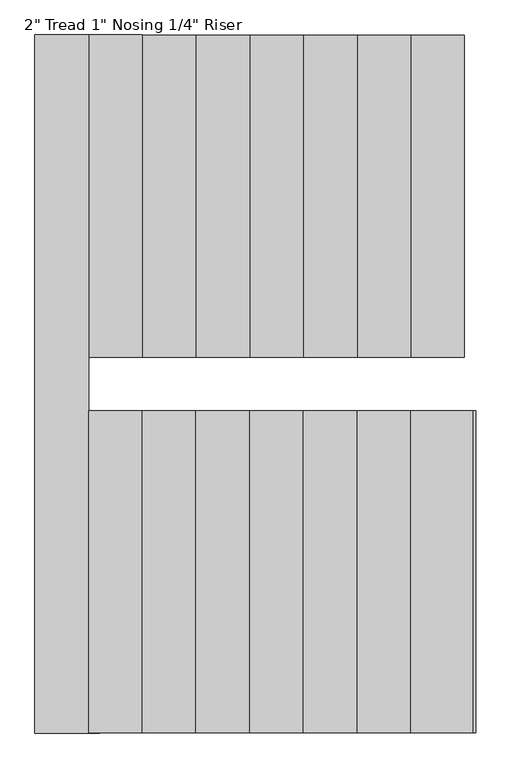
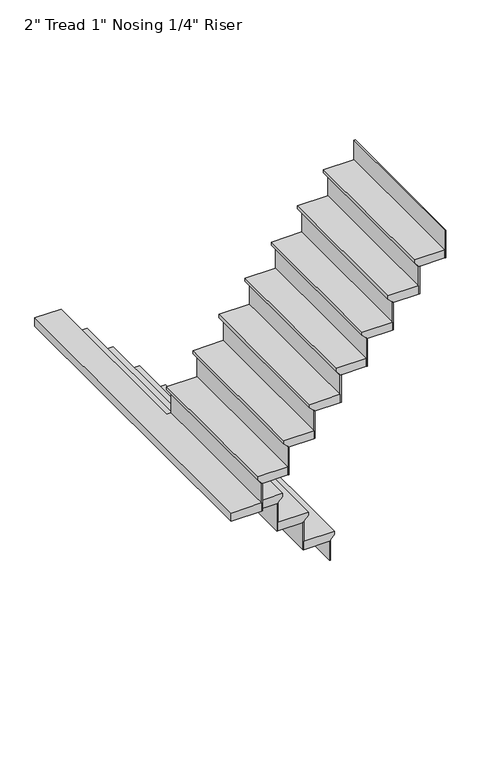
"""IFC4 building model written with IfcOpenShell, lengths in millimetres: stair flight geometry."""

from ifc_helpers import new_model, si_unit, origin, place, context, project, spatial, faceted_brep, source, transform, mapped, element, save


def stair_flight_9f5b5764(model_context):
    return source(origin(), model_context, "Body", "Brep", [
        faceted_brep([(3632.2, 10909.3, 9294.2833333), (3632.2, 10909.3, 9313.3333333), (3632.2, 9994.9, 9313.3333333), (3632.2, 9994.9, 9294.2833333), (3606.8, 10909.3, 9268.8833333), (3606.8, 9994.9, 9268.8833333), (3454.4, 10909.3, 9313.3333333), (3454.4, 9994.9, 9313.3333333), (3606.8, 9994.9, 9262.5333333), (3454.4, 9994.9, 9262.5333333), (3454.4, 10909.3, 9262.5333333), (3606.8, 10909.3, 9262.5333333)], [[[0, 1, 2, 3]], [[4, 0, 3, 5]], [[2, 1, 6, 7]], [[8, 9, 10, 11]], [[2, 7, 9, 8, 5, 3]], [[8, 11, 4, 5]], [[6, 1, 0, 4, 11, 10]], [[7, 6, 10, 9]]]),
        faceted_brep([(3606.8, 10909.3, 9262.5333333), (3606.8, 10909.3, 9144.0), (3600.45, 10909.3, 9144.0), (3600.45, 10909.3, 9262.5333333), (3606.8, 9994.9, 9262.5333333), (3600.45, 9994.9, 9262.5333333), (3600.45, 9994.9, 9144.0), (3606.8, 9994.9, 9144.0)], [[[0, 1, 2, 3]], [[4, 5, 6, 7]], [[1, 0, 4, 7]], [[2, 1, 7, 6]], [[3, 2, 6, 5]], [[0, 3, 5, 4]]]),
        faceted_brep([(3454.4, 10909.3, 9431.8666667), (3454.4, 10909.3, 9262.5333333), (3448.05, 10909.3, 9262.5333333), (3448.05, 10909.3, 9431.8666667), (3454.4, 9994.9, 9431.8666667), (3448.05, 9994.9, 9431.8666667), (3448.05, 9994.9, 9262.5333333), (3454.4, 9994.9, 9262.5333333)], [[[0, 1, 2, 3]], [[4, 5, 6, 7]], [[1, 0, 4, 7]], [[2, 1, 7, 6]], [[3, 2, 6, 5]], [[0, 3, 5, 4]]]),
        faceted_brep([(3479.8, 9994.9, 9482.6666667), (3479.8, 10909.3, 9482.6666667), (3302.0, 10909.3, 9482.6666667), (3302.0, 9994.9, 9482.6666667), (3454.4, 9994.9, 9431.8666667), (3302.0, 9994.9, 9431.8666667), (3302.0, 10909.3, 9431.8666667), (3454.4, 10909.3, 9431.8666667), (3454.4, 9994.9, 9438.2166667), (3479.8, 9994.9, 9463.6166667), (3454.4, 10909.3, 9438.2166667), (3479.8, 10909.3, 9463.6166667)], [[[0, 1, 2, 3]], [[4, 5, 6, 7]], [[0, 3, 5, 4, 8, 9]], [[4, 7, 10, 8]], [[2, 1, 11, 10, 7, 6]], [[3, 2, 6, 5]], [[11, 1, 0, 9]], [[10, 11, 9, 8]]]),
        faceted_brep([(3302.0, 10909.3, 9601.2), (3302.0, 10909.3, 9431.8666667), (3295.65, 10909.3, 9431.8666667), (3295.65, 10909.3, 9601.2), (3302.0, 9994.9, 9601.2), (3295.65, 9994.9, 9601.2), (3295.65, 9994.9, 9431.8666667), (3302.0, 9994.9, 9431.8666667)], [[[0, 1, 2, 3]], [[4, 5, 6, 7]], [[1, 0, 4, 7]], [[2, 1, 7, 6]], [[3, 2, 6, 5]], [[0, 3, 5, 4]]]),
        faceted_brep([(3327.4, 9994.9, 9652.0), (3327.4, 10909.3, 9652.0), (3149.6, 10909.3, 9652.0), (3149.6, 9994.9, 9652.0), (3302.0, 9994.9, 9601.2), (3149.6, 9994.9, 9601.2), (3149.6, 10909.3, 9601.2), (3302.0, 10909.3, 9601.2), (3302.0, 9994.9, 9607.55), (3327.4, 9994.9, 9632.95), (3302.0, 10909.3, 9607.55), (3327.4, 10909.3, 9632.95)], [[[0, 1, 2, 3]], [[4, 5, 6, 7]], [[0, 3, 5, 4, 8, 9]], [[4, 7, 10, 8]], [[2, 1, 11, 10, 7, 6]], [[3, 2, 6, 5]], [[11, 1, 0, 9]], [[10, 11, 9, 8]]]),
        faceted_brep([(3149.6, 10909.3, 9770.5333333), (3149.6, 10909.3, 9601.2), (3143.25, 10909.3, 9601.2), (3143.25, 10909.3, 9770.5333333), (3149.6, 9994.9, 9770.5333333), (3143.25, 9994.9, 9770.5333333), (3143.25, 9994.9, 9601.2), (3149.6, 9994.9, 9601.2)], [[[0, 1, 2, 3]], [[4, 5, 6, 7]], [[1, 0, 4, 7]], [[2, 1, 7, 6]], [[3, 2, 6, 5]], [[0, 3, 5, 4]]]),
        faceted_brep([(3175.0, 9994.9, 9821.3333333), (3175.0, 10909.3, 9821.3333333), (2997.2, 10909.3, 9821.3333333), (2997.2, 9994.9, 9821.3333333), (3149.6, 9994.9, 9770.5333333), (2997.2, 9994.9, 9770.5333333), (2997.2, 10909.3, 9770.5333333), (3149.6, 10909.3, 9770.5333333), (3149.6, 9994.9, 9776.8833333), (3175.0, 9994.9, 9802.2833333), (3149.6, 10909.3, 9776.8833333), (3175.0, 10909.3, 9802.2833333)], [[[0, 1, 2, 3]], [[4, 5, 6, 7]], [[0, 3, 5, 4, 8, 9]], [[4, 7, 10, 8]], [[2, 1, 11, 10, 7, 6]], [[3, 2, 6, 5]], [[11, 1, 0, 9]], [[10, 11, 9, 8]]]),
        faceted_brep([(2997.2, 10909.3, 9939.8666667), (2997.2, 10909.3, 9770.5333333), (2990.85, 10909.3, 9770.5333333), (2990.85, 10909.3, 9939.8666667), (2997.2, 9994.9, 9939.8666667), (2990.85, 9994.9, 9939.8666667), (2990.85, 9994.9, 9770.5333333), (2997.2, 9994.9, 9770.5333333)], [[[0, 1, 2, 3]], [[4, 5, 6, 7]], [[1, 0, 4, 7]], [[2, 1, 7, 6]], [[3, 2, 6, 5]], [[0, 3, 5, 4]]]),
        faceted_brep([(3022.6, 9994.9, 9990.6666667), (3022.6, 10909.3, 9990.6666667), (2844.8, 10909.3, 9990.6666667), (2844.8, 9994.9, 9990.6666667), (2997.2, 9994.9, 9939.8666667), (2844.8, 9994.9, 9939.8666667), (2844.8, 10909.3, 9939.8666667), (2997.2, 10909.3, 9939.8666667), (2997.2, 9994.9, 9946.2166667), (3022.6, 9994.9, 9971.6166667), (2997.2, 10909.3, 9946.2166667), (3022.6, 10909.3, 9971.6166667)], [[[0, 1, 2, 3]], [[4, 5, 6, 7]], [[0, 3, 5, 4, 8, 9]], [[4, 7, 10, 8]], [[2, 1, 11, 10, 7, 6]], [[3, 2, 6, 5]], [[11, 1, 0, 9]], [[10, 11, 9, 8]]]),
        faceted_brep([(2844.8, 10909.3, 10109.2), (2844.8, 10909.3, 9939.8666667), (2838.45, 10909.3, 9939.8666667), (2838.45, 10909.3, 10109.2), (2844.8, 9994.9, 10109.2), (2838.45, 9994.9, 10109.2), (2838.45, 9994.9, 9939.8666667), (2844.8, 9994.9, 9939.8666667)], [[[0, 1, 2, 3]], [[4, 5, 6, 7]], [[1, 0, 4, 7]], [[2, 1, 7, 6]], [[3, 2, 6, 5]], [[0, 3, 5, 4]]]),
        faceted_brep([(2870.2, 9994.9, 10160.0), (2870.2, 10909.3, 10160.0), (2692.4, 10909.3, 10160.0), (2692.4, 9994.9, 10160.0), (2844.8, 9994.9, 10109.2), (2692.4, 9994.9, 10109.2), (2692.4, 10909.3, 10109.2), (2844.8, 10909.3, 10109.2), (2844.8, 9994.9, 10115.55), (2870.2, 9994.9, 10140.95), (2844.8, 10909.3, 10115.55), (2870.2, 10909.3, 10140.95)], [[[0, 1, 2, 3]], [[4, 5, 6, 7]], [[0, 3, 5, 4, 8, 9]], [[4, 7, 10, 8]], [[2, 1, 11, 10, 7, 6]], [[3, 2, 6, 5]], [[11, 1, 0, 9]], [[10, 11, 9, 8]]]),
        faceted_brep([(2692.4, 10909.3, 10278.5333333), (2692.4, 10909.3, 10109.2), (2686.05, 10909.3, 10109.2), (2686.05, 10909.3, 10278.5333333), (2692.4, 9994.9, 10278.5333333), (2686.05, 9994.9, 10278.5333333), (2686.05, 9994.9, 10109.2), (2692.4, 9994.9, 10109.2)], [[[0, 1, 2, 3]], [[4, 5, 6, 7]], [[1, 0, 4, 7]], [[2, 1, 7, 6]], [[3, 2, 6, 5]], [[0, 3, 5, 4]]]),
        faceted_brep([(2717.8, 9994.9, 10329.3333333), (2717.8, 10909.3, 10329.3333333), (2540.0, 10909.3, 10329.3333333), (2540.0, 9994.9, 10329.3333333), (2692.4, 9994.9, 10278.5333333), (2540.0, 9994.9, 10278.5333333), (2540.0, 10909.3, 10278.5333333), (2692.4, 10909.3, 10278.5333333), (2692.4, 9994.9, 10284.8833333), (2717.8, 9994.9, 10310.2833333), (2692.4, 10909.3, 10284.8833333), (2717.8, 10909.3, 10310.2833333)], [[[0, 1, 2, 3]], [[4, 5, 6, 7]], [[0, 3, 5, 4, 8, 9]], [[4, 7, 10, 8]], [[2, 1, 11, 10, 7, 6]], [[3, 2, 6, 5]], [[11, 1, 0, 9]], [[10, 11, 9, 8]]]),
        faceted_brep([(2540.0, 10909.3, 10447.8666667), (2540.0, 10909.3, 10278.5333333), (2533.65, 10909.3, 10278.5333333), (2533.65, 10909.3, 10447.8666667), (2540.0, 9994.9, 10447.8666667), (2533.65, 9994.9, 10447.8666667), (2533.65, 9994.9, 10278.5333333), (2540.0, 9994.9, 10278.5333333)], [[[0, 1, 2, 3]], [[4, 5, 6, 7]], [[1, 0, 4, 7]], [[2, 1, 7, 6]], [[3, 2, 6, 5]], [[0, 3, 5, 4]]]),
        faceted_brep([(2590.8, 9842.5, 10498.6666667), (2565.4, 9842.5, 10498.6666667), (2565.4, 10909.3, 10498.6666667), (2413.0, 10909.3, 10498.6666667), (2413.0, 8928.1, 10498.6666667), (2590.8, 8928.1, 10498.6666667), (2565.4, 9842.5, 10447.8666667), (2590.8, 9842.5, 10447.8666667), (2590.8, 8928.1, 10447.8666667), (2413.0, 8928.1, 10447.8666667), (2413.0, 10909.3, 10447.8666667), (2540.0, 10909.3, 10447.8666667), (2540.0, 9994.9, 10447.8666667), (2565.4, 9994.9, 10447.8666667), (2565.4, 9994.9, 10479.6166667), (2565.4, 10909.3, 10479.6166667), (2540.0, 9994.9, 10454.2166667), (2540.0, 10909.3, 10454.2166667)], [[[0, 1, 2, 3, 4, 5]], [[6, 7, 8, 9, 10, 11, 12, 13]], [[1, 0, 7, 6]], [[2, 1, 6, 13, 14, 15]], [[13, 12, 16, 14]], [[12, 11, 17, 16]], [[3, 2, 15, 17, 11, 10]], [[4, 3, 10, 9]], [[5, 4, 9, 8]], [[0, 5, 8, 7]], [[17, 15, 14, 16]]]),
        faceted_brep([(2590.8, 8928.1, 10617.2), (2590.8, 8928.1, 10447.8666667), (2597.15, 8928.1, 10447.8666667), (2597.15, 8928.1, 10617.2), (2590.8, 9842.5, 10617.2), (2597.15, 9842.5, 10617.2), (2597.15, 9842.5, 10447.8666667), (2590.8, 9842.5, 10447.8666667)], [[[0, 1, 2, 3]], [[4, 5, 6, 7]], [[1, 0, 4, 7]], [[2, 1, 7, 6]], [[3, 2, 6, 5]], [[0, 3, 5, 4]]]),
        faceted_brep([(2565.4, 9842.5, 10668.0), (2565.4, 8928.1, 10668.0), (2743.2, 8928.1, 10668.0), (2743.2, 9842.5, 10668.0), (2590.8, 9842.5, 10617.2), (2743.2, 9842.5, 10617.2), (2743.2, 8928.1, 10617.2), (2590.8, 8928.1, 10617.2), (2590.8, 9842.5, 10623.55), (2565.4, 9842.5, 10648.95), (2590.8, 8928.1, 10623.55), (2565.4, 8928.1, 10648.95)], [[[0, 1, 2, 3]], [[4, 5, 6, 7]], [[0, 3, 5, 4, 8, 9]], [[4, 7, 10, 8]], [[2, 1, 11, 10, 7, 6]], [[3, 2, 6, 5]], [[11, 1, 0, 9]], [[10, 11, 9, 8]]]),
        faceted_brep([(2743.2, 8928.1, 10786.5333333), (2743.2, 8928.1, 10617.2), (2749.55, 8928.1, 10617.2), (2749.55, 8928.1, 10786.5333333), (2743.2, 9842.5, 10786.5333333), (2749.55, 9842.5, 10786.5333333), (2749.55, 9842.5, 10617.2), (2743.2, 9842.5, 10617.2)], [[[0, 1, 2, 3]], [[4, 5, 6, 7]], [[1, 0, 4, 7]], [[2, 1, 7, 6]], [[3, 2, 6, 5]], [[0, 3, 5, 4]]]),
        faceted_brep([(2717.8, 9842.5, 10837.3333333), (2717.8, 8928.1, 10837.3333333), (2895.6, 8928.1, 10837.3333333), (2895.6, 9842.5, 10837.3333333), (2743.2, 9842.5, 10786.5333333), (2895.6, 9842.5, 10786.5333333), (2895.6, 8928.1, 10786.5333333), (2743.2, 8928.1, 10786.5333333), (2743.2, 9842.5, 10792.8833333), (2717.8, 9842.5, 10818.2833333), (2743.2, 8928.1, 10792.8833333), (2717.8, 8928.1, 10818.2833333)], [[[0, 1, 2, 3]], [[4, 5, 6, 7]], [[0, 3, 5, 4, 8, 9]], [[4, 7, 10, 8]], [[2, 1, 11, 10, 7, 6]], [[3, 2, 6, 5]], [[11, 1, 0, 9]], [[10, 11, 9, 8]]]),
        faceted_brep([(2895.6, 8928.1, 10955.8666667), (2895.6, 8928.1, 10786.5333333), (2901.95, 8928.1, 10786.5333333), (2901.95, 8928.1, 10955.8666667), (2895.6, 9842.5, 10955.8666667), (2901.95, 9842.5, 10955.8666667), (2901.95, 9842.5, 10786.5333333), (2895.6, 9842.5, 10786.5333333)], [[[0, 1, 2, 3]], [[4, 5, 6, 7]], [[1, 0, 4, 7]], [[2, 1, 7, 6]], [[3, 2, 6, 5]], [[0, 3, 5, 4]]]),
        faceted_brep([(2870.2, 9842.5, 11006.6666667), (2870.2, 8928.1, 11006.6666667), (3048.0, 8928.1, 11006.6666667), (3048.0, 9842.5, 11006.6666667), (2895.6, 9842.5, 10955.8666667), (3048.0, 9842.5, 10955.8666667), (3048.0, 8928.1, 10955.8666667), (2895.6, 8928.1, 10955.8666667), (2895.6, 9842.5, 10962.2166667), (2870.2, 9842.5, 10987.6166667), (2895.6, 8928.1, 10962.2166667), (2870.2, 8928.1, 10987.6166667)], [[[0, 1, 2, 3]], [[4, 5, 6, 7]], [[0, 3, 5, 4, 8, 9]], [[4, 7, 10, 8]], [[2, 1, 11, 10, 7, 6]], [[3, 2, 6, 5]], [[11, 1, 0, 9]], [[10, 11, 9, 8]]]),
        faceted_brep([(3048.0, 8928.1, 11125.2), (3048.0, 8928.1, 10955.8666667), (3054.35, 8928.1, 10955.8666667), (3054.35, 8928.1, 11125.2), (3048.0, 9842.5, 11125.2), (3054.35, 9842.5, 11125.2), (3054.35, 9842.5, 10955.8666667), (3048.0, 9842.5, 10955.8666667)], [[[0, 1, 2, 3]], [[4, 5, 6, 7]], [[1, 0, 4, 7]], [[2, 1, 7, 6]], [[3, 2, 6, 5]], [[0, 3, 5, 4]]]),
        faceted_brep([(3022.6, 9842.5, 11176.0), (3022.6, 8928.1, 11176.0), (3200.4, 8928.1, 11176.0), (3200.4, 9842.5, 11176.0), (3048.0, 9842.5, 11125.2), (3200.4, 9842.5, 11125.2), (3200.4, 8928.1, 11125.2), (3048.0, 8928.1, 11125.2), (3048.0, 9842.5, 11131.55), (3022.6, 9842.5, 11156.95), (3048.0, 8928.1, 11131.55), (3022.6, 8928.1, 11156.95)], [[[0, 1, 2, 3]], [[4, 5, 6, 7]], [[0, 3, 5, 4, 8, 9]], [[4, 7, 10, 8]], [[2, 1, 11, 10, 7, 6]], [[3, 2, 6, 5]], [[11, 1, 0, 9]], [[10, 11, 9, 8]]]),
        faceted_brep([(3200.4, 8928.1, 11294.5333333), (3200.4, 8928.1, 11125.2), (3206.75, 8928.1, 11125.2), (3206.75, 8928.1, 11294.5333333), (3200.4, 9842.5, 11294.5333333), (3206.75, 9842.5, 11294.5333333), (3206.75, 9842.5, 11125.2), (3200.4, 9842.5, 11125.2)], [[[0, 1, 2, 3]], [[4, 5, 6, 7]], [[1, 0, 4, 7]], [[2, 1, 7, 6]], [[3, 2, 6, 5]], [[0, 3, 5, 4]]]),
        faceted_brep([(3175.0, 9842.5, 11345.3333333), (3175.0, 8928.1, 11345.3333333), (3352.8, 8928.1, 11345.3333333), (3352.8, 9842.5, 11345.3333333), (3200.4, 9842.5, 11294.5333333), (3352.8, 9842.5, 11294.5333333), (3352.8, 8928.1, 11294.5333333), (3200.4, 8928.1, 11294.5333333), (3200.4, 9842.5, 11300.8833333), (3175.0, 9842.5, 11326.2833333), (3200.4, 8928.1, 11300.8833333), (3175.0, 8928.1, 11326.2833333)], [[[0, 1, 2, 3]], [[4, 5, 6, 7]], [[0, 3, 5, 4, 8, 9]], [[4, 7, 10, 8]], [[2, 1, 11, 10, 7, 6]], [[3, 2, 6, 5]], [[11, 1, 0, 9]], [[10, 11, 9, 8]]]),
        faceted_brep([(3352.8, 8928.1, 11463.8666667), (3352.8, 8928.1, 11294.5333333), (3359.15, 8928.1, 11294.5333333), (3359.15, 8928.1, 11463.8666667), (3352.8, 9842.5, 11463.8666667), (3359.15, 9842.5, 11463.8666667), (3359.15, 9842.5, 11294.5333333), (3352.8, 9842.5, 11294.5333333)], [[[0, 1, 2, 3]], [[4, 5, 6, 7]], [[1, 0, 4, 7]], [[2, 1, 7, 6]], [[3, 2, 6, 5]], [[0, 3, 5, 4]]]),
        faceted_brep([(3327.4, 9842.5, 11514.6666667), (3327.4, 8928.1, 11514.6666667), (3505.2, 8928.1, 11514.6666667), (3505.2, 9842.5, 11514.6666667), (3352.8, 9842.5, 11463.8666667), (3505.2, 9842.5, 11463.8666667), (3505.2, 8928.1, 11463.8666667), (3352.8, 8928.1, 11463.8666667), (3352.8, 9842.5, 11470.2166667), (3327.4, 9842.5, 11495.6166667), (3352.8, 8928.1, 11470.2166667), (3327.4, 8928.1, 11495.6166667)], [[[0, 1, 2, 3]], [[4, 5, 6, 7]], [[0, 3, 5, 4, 8, 9]], [[4, 7, 10, 8]], [[2, 1, 11, 10, 7, 6]], [[3, 2, 6, 5]], [[11, 1, 0, 9]], [[10, 11, 9, 8]]]),
        faceted_brep([(3505.2, 8928.1, 11633.2), (3505.2, 8928.1, 11463.8666667), (3511.55, 8928.1, 11463.8666667), (3511.55, 8928.1, 11633.2), (3505.2, 9842.5, 11633.2), (3511.55, 9842.5, 11633.2), (3511.55, 9842.5, 11463.8666667), (3505.2, 9842.5, 11463.8666667)], [[[0, 1, 2, 3]], [[4, 5, 6, 7]], [[1, 0, 4, 7]], [[2, 1, 7, 6]], [[3, 2, 6, 5]], [[0, 3, 5, 4]]]),
        faceted_brep([(3657.6, 8928.1, 11802.5333333), (3657.6, 8928.1, 11633.2), (3663.95, 8928.1, 11633.2), (3663.95, 8928.1, 11802.5333333), (3657.6, 9842.5, 11802.5333333), (3663.95, 9842.5, 11802.5333333), (3663.95, 9842.5, 11633.2), (3657.6, 9842.5, 11633.2)], [[[0, 1, 2, 3]], [[4, 5, 6, 7]], [[1, 0, 4, 7]], [[2, 1, 7, 6]], [[3, 2, 6, 5]], [[0, 3, 5, 4]]]),
        faceted_brep([(3479.8, 9842.5, 11684.0), (3479.8, 8928.1, 11684.0), (3657.6, 8928.1, 11684.0), (3657.6, 9842.5, 11684.0), (3505.2, 9842.5, 11633.2), (3657.6, 9842.5, 11633.2), (3657.6, 8928.1, 11633.2), (3505.2, 8928.1, 11633.2), (3505.2, 9842.5, 11639.55), (3479.8, 9842.5, 11664.95), (3505.2, 8928.1, 11639.55), (3479.8, 8928.1, 11664.95)], [[[0, 1, 2, 3]], [[4, 5, 6, 7]], [[0, 3, 5, 4, 8, 9]], [[4, 7, 10, 8]], [[2, 1, 11, 10, 7, 6]], [[3, 2, 6, 5]], [[11, 1, 0, 9]], [[10, 11, 9, 8]]]),
    ])


if __name__ == "__main__":
    model = new_model("IFC4")
    model_context = context("Model", 3, world=origin())
    ifc_project = project(units=[si_unit("LENGTHUNIT", "METRE", prefix="MILLI")], contexts=[model_context])
    site = spatial("IfcSite", under=ifc_project)
    building = spatial("IfcBuilding", under=site)
    placement = place(None, origin())
    stair_flight_shape = stair_flight_9f5b5764(model_context)
    element("IfcStairFlight", 1, ObjectType="2\" Tread 1\" Nosing 1/4\" Riser", at=placement, inside=building, context=model_context, shape_type="MappedRepresentation", body=[
        mapped(stair_flight_shape, transform((0.0, 0.0, 0.0), x_axis=(1.0, 0.0, 0.0), y_axis=(0.0, 1.0, 0.0), z_axis=(0.0, 0.0, 1.0))),
    ])
    save(model, "model.ifc")
